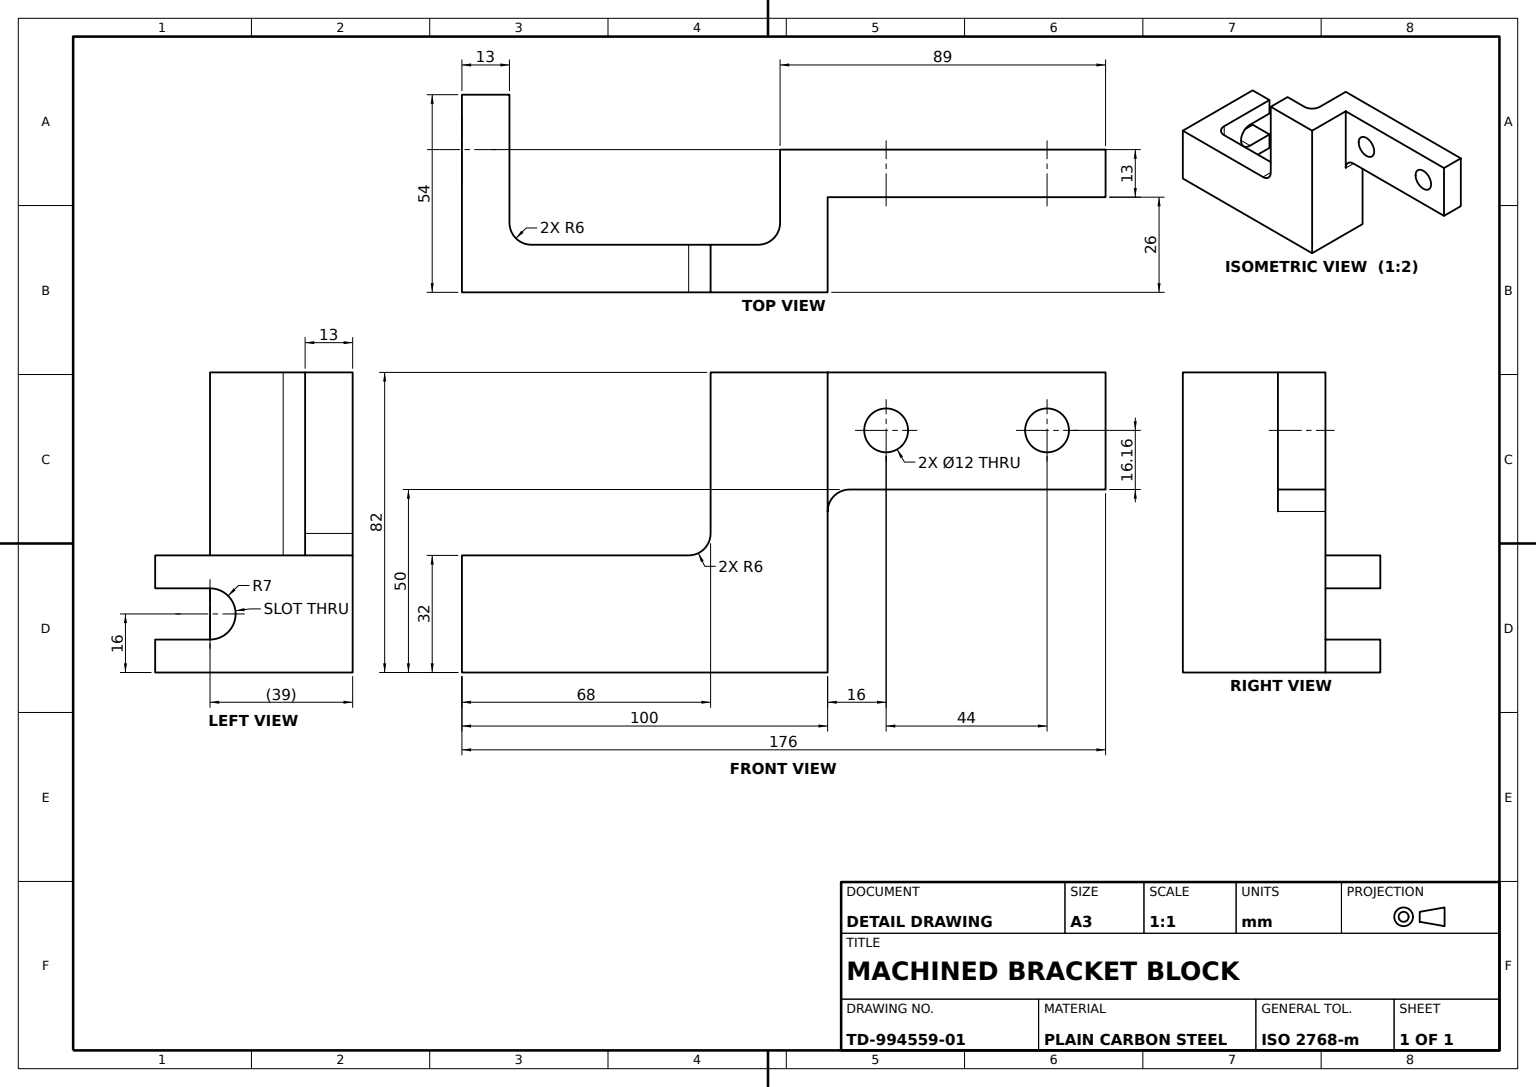
from build123d import *

# Parameters (mm, degrees)
BASE_PROFILE_13MM_DEPTH    = 13
UPRIGHT_BLOCK_82MM_DEPTH   = 82
RECTANGULAR_CUT_SKETCH_W   = 54
RECTANGULAR_CUT_SKETCH_H   = 50
RECTANGULAR_CUT_20MM_DEPTH = 20
POCKET_CUT_SKETCH_W        = 13
POCKET_CUT_SKETCH_H        = 32
POCKET_CUT_13MM_DEPTH      = 13
SLOT_CUT_14MM_DEPTH        = 13
MOUNTING_FLANGE_6MM_DEPTH  = 13
FLANGE_HOLES_SKETCH_R      = 6
FLANGE_HOLES_2X_12_DEPTH   = 13


with BuildPart() as part:
    # Base Profile Sketch → Base Profile 13mm (new body)
    with BuildSketch(Plane.XY):
        with BuildLine():
            Line((0, 0), (100, 0))
            Line((100, 0), (100, 82))
            Line((100, 82), (68, 82))
            Line((68, 82), (68, 38))
            ThreePointArc((68, 38), (66.242640687, 33.757359313), (62, 32))
            Line((62, 32), (0, 32))
            Line((0, 32), (0, 0))
        make_face()
    extrude(amount=BASE_PROFILE_13MM_DEPTH)

    # Upright Block Sketch → Upright Block 82mm (add)
    with BuildSketch(Plane.XZ):
        with BuildLine():
            Line((19, 0), (0, 0))
            Line((0, 0), (0, -54))
            Line((0, -54), (13, -54))
            Line((13, -54), (13, -6))
            ThreePointArc((13, -6), (14.757359313, -1.757359313), (19, 0))
        make_face()
        with BuildLine():
            Line((100, 0), (81, 0))
            ThreePointArc((81, 0), (85.242640687, -1.757359313), (87, -6))
            Line((87, -6), (87, -26))
            Line((87, -26), (100, -26))
            Line((100, -26), (100, 0))
        make_face()
    extrude(amount=-UPRIGHT_BLOCK_82MM_DEPTH)

    # Rectangular Cut Sketch → Rectangular Cut 20mm (cut)
    with BuildSketch(Plane.ZY):
        with Locations((-27, 57)):
            Rectangle(RECTANGULAR_CUT_SKETCH_W, RECTANGULAR_CUT_SKETCH_H)
    extrude(amount=-RECTANGULAR_CUT_20MM_DEPTH, mode=Mode.SUBTRACT)

    # Pocket Cut Sketch → Pocket Cut 13mm (cut)
    with BuildSketch(Plane(origin=(0, 0, -54), x_dir=(-1, 0, 0), z_dir=(0, 0, -1))):
        with Locations((-6.5, 16)):
            Rectangle(POCKET_CUT_SKETCH_W, POCKET_CUT_SKETCH_H)
    extrude(amount=-POCKET_CUT_13MM_DEPTH, mode=Mode.SUBTRACT)

    # Slot Cut Sketch → Slot Cut 14mm (cut)
    with BuildSketch(Plane.ZY):
        with BuildLine():
            Line((-41, 9), (-26, 9))
            ThreePointArc((-26, 9), (-19, 16), (-26, 23))
            Line((-26, 23), (-41, 23))
            Line((-41, 23), (-41, 9))
        make_face()
    extrude(amount=-SLOT_CUT_14MM_DEPTH, mode=Mode.SUBTRACT)

    # Mounting Flange Sketch → Mounting Flange 6mm (add)
    with BuildSketch(Plane(origin=(0, 0, -26), x_dir=(-1, 0, 0), z_dir=(0, 0, -1))):
        with BuildLine():
            Line((-100, 82), (-176, 82))
            Line((-176, 82), (-176, 50))
            Line((-176, 50), (-106, 50))
            ThreePointArc((-106, 50), (-101.757359313, 48.242640687), (-100, 44))
            Line((-100, 44), (-100, 82))
        make_face()
    extrude(amount=-MOUNTING_FLANGE_6MM_DEPTH)

    # Flange Holes Sketch → Flange Holes 2xØ12 (cut)
    with BuildSketch(Plane.XY.offset(-13)):
        with Locations((116, 66.156876682)):
            Circle(FLANGE_HOLES_SKETCH_R)
        with Locations((160, 66.156876682)):
            Circle(FLANGE_HOLES_SKETCH_R)
    extrude(amount=-FLANGE_HOLES_2X_12_DEPTH, mode=Mode.SUBTRACT)


solid = part.part
